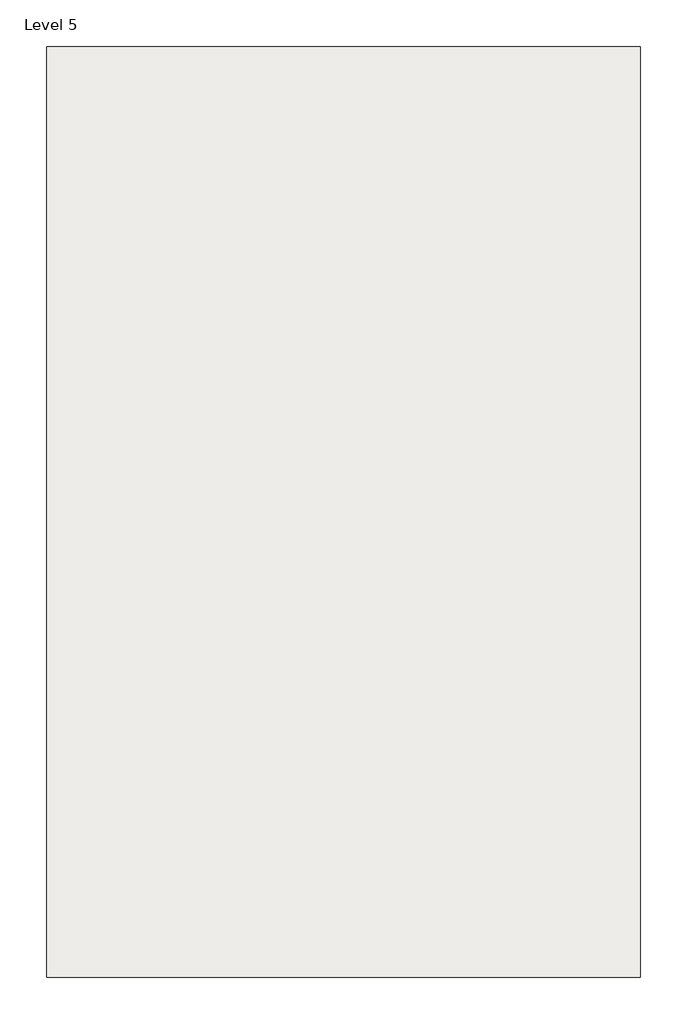
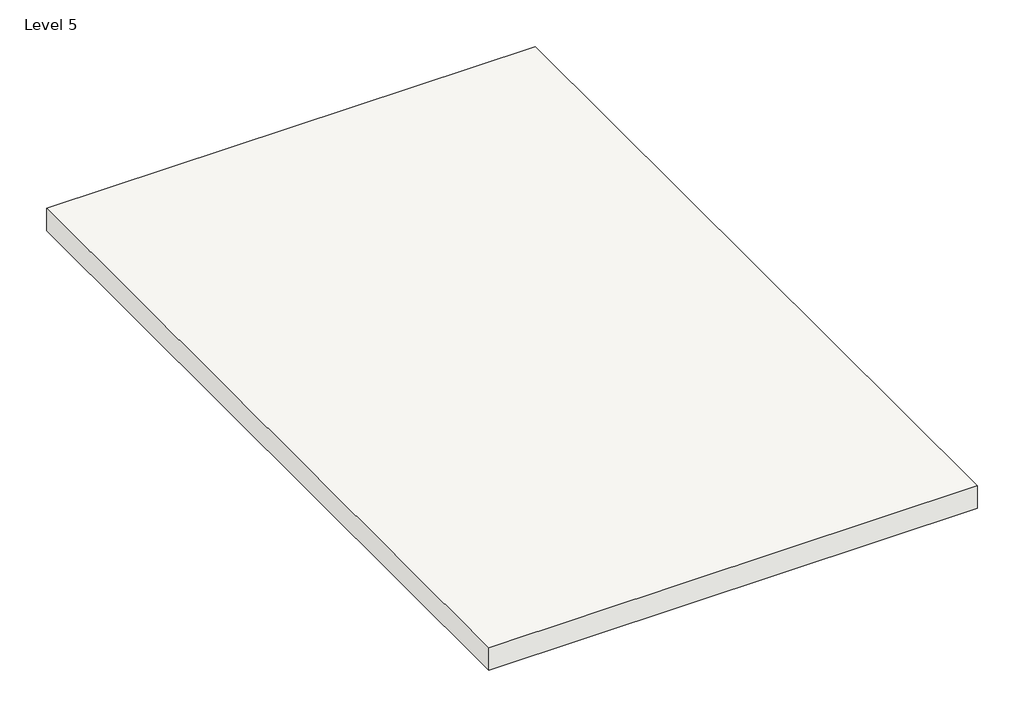
# One storey: 1 slab.
"""IFC4 building model written with IfcOpenShell, lengths in millimetres."""

from ifc_helpers import new_model, si_unit, frame, origin, place, context, project, spatial, polyline, outline, extrude, element, save

model = new_model("IFC4")

# Units and contexts
model_context = context("Model", 3, world=origin())
ifc_project = project(units=[si_unit("LENGTHUNIT", "METRE", prefix="MILLI")], contexts=[model_context])

# Site, building, storey
site = spatial("IfcSite", under=ifc_project)
building = spatial("IfcBuilding", under=site)
storey = spatial("IfcBuildingStorey", under=building, Name="Level 5", Elevation=12192.0)

# Slab
placement = place(None, origin())
element("IfcSlab", 1, ObjectType="6\" FLOOR", at=placement, inside=storey, context=model_context, shape_type="SweptSolid", body=[
    extrude(outline(polyline([(392.0391502, 5370.1115866), (392.0391502, 428.4115866), (-2760.3608498, 428.4115866), (-2760.3608498, 5370.1115866), (392.0391502, 5370.1115866)])), frame((0.0, 0.0, 9144.0), z_axis=(0.0, 0.0, 1.0), x_axis=(1.0, 0.0, 0.0)), (0.0, 0.0, 1.0), 152.4),
])

save(model, "model.ifc")

# Revit data of these elements
# Type "6\" FLOOR"
#   Assembly Code = "B1010"
#   Function = 0
#   Layers, outside or top first: 0' - 6" no material (function 1)
# Element 1 (IfcSlab, "6\" FLOOR")
#   built-in parameter 1001955 = 3.14159 (stored number, unit not read)
#   Height Offset From Level = -9' - 6"
#   Phase Created = New Construction
#   Materials on its faces: "Default Floor"
# Materials
#   "Default Floor": colour RGB 128 128 128, transparency 0, Cost = 0
